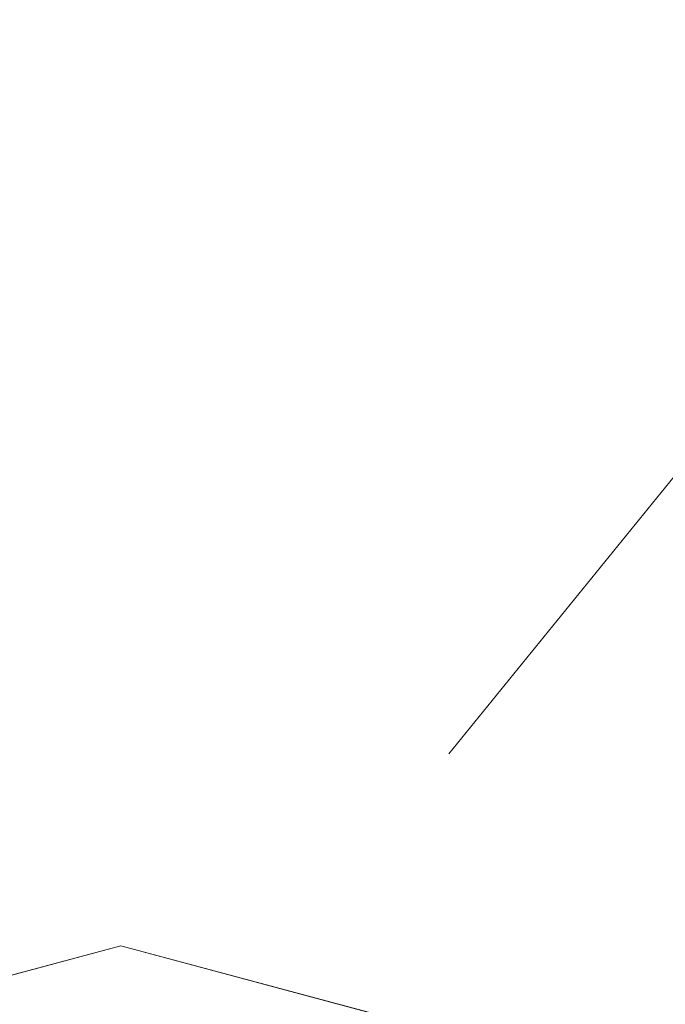
# Model space of a CAD drawing. Units: inches. Extents: x 375 to 1122, y 27 to 1069.
# Tile 89 of 155: x 725.203 to 728.243, y 859.033 to 863.668. Entities that reach past the tile are written whole.
import ezdxf

# ---------------------------------------------------------------- set-up
doc = ezdxf.new("R2010")
doc.units = ezdxf.units.IN
doc.layers.add('A-ANNO-DIMS', color=2, linetype='Continuous', lineweight=18)
doc.layers.add('Furniture', color=30, linetype='Continuous', lineweight=18)
doc.styles.get("Standard").update_dxf_attribs({"font": 'arial.ttf'})
doc.dimstyles.new('ISO-25', dxfattribs={"dimtxt": 12, "dimasz": 2.5, "dimexe": 1.5, "dimexo": 1.5, "dimtad": 1, "dimdec": 1, "dimlunit": 3, "dimtxsty": 'Standard', "dimblk": 'ARCHTICK', "dimcen": 2.5, "dimadec": 0, "dimazin": 0, "dimtfac": 1, "dimtdec": 1, "dimtmove": 0, "dimatfit": 3, "dimfxl": 1.5, "dimfxlon": 1, "dimarcsym": 0})

# ---------------------------------------------------------------- blocks, each defined once
blk = doc.blocks.new('A$C403C54AD')
blk.add_line((1.78922, 1.18993, 0.03663), (1.95298, 1.05694, 0.03663))
at = {"linetype": 'ByBlock', "invisible_edges": 5}
for points in [[(1.99415, 1.08761, -0.03783), (2.01014, 1.07837, -0.03783), (1.99406, 1.01834, -0.03783), (1.97559, 1.01834, -0.03783)], [(2.02347, 1.07068, -0.05168), (1.99415, 1.08761, -0.04244), (1.97559, 1.01834, -0.04244), (2.00945, 1.01834, -0.05168)], [(1.97559, 1.01834, -0.03783), (1.99406, 1.01834, -0.03783), (2.01014, 0.95832, -0.03783), (1.99415, 0.94908, -0.03783)], [(2.00945, 1.01834, -0.05168), (1.97559, 1.01834, -0.04244), (1.99415, 0.94908, -0.04244), (2.02347, 0.96601, -0.05168)]]:
    blk.add_3dface(points, dxfattribs=at)
at = {"linetype": 'ByBlock'}
for points in [[(1.99415, 1.08761, -0.04244), (1.99415, 1.08761, -0.03783), (1.97559, 1.01834, -0.03783), (1.97559, 1.01834, -0.04244)], [(1.97559, 1.01834, -0.04244), (1.97559, 1.01834, -0.03783), (1.99415, 0.94908, -0.03783), (1.99415, 0.94908, -0.04244)]]:
    blk.add_3dface(points, dxfattribs=at)
blk = doc.blocks.new('_ArchTick')
at = {"color": 0, "linetype": 'ByBlock', "const_width": 0.15}
blk.add_lwpolyline([(-0.5, -0.5), (0.5, 0.5)], dxfattribs=at)
blk = doc.blocks.new('*D85')
at = {"layer": 'A-ANNO-DIMS', "color": 0, "lineweight": -2, "transparency": 16777216}
for p, q in [((401.5073, 868.5277), (398.5073, 868.5277)), ((400.0073, 814.5277), (400.0073, 868.5277)), ((401.5073, 814.5277), (398.5073, 814.5277))]:
    blk.add_line(p, q, dxfattribs=at)
at = {"layer": 'Defpoints', "color": 0, "transparency": 16777216}
for p in [(400.0073, 868.5277), (845.0073, 868.5277), (845.0073, 814.5277)]:
    blk.add_point(p, dxfattribs=at)
at = {"layer": 'A-ANNO-DIMS', "color": 0, "lineweight": -2, "transparency": 16777216, "xscale": 2.5, "yscale": 2.5, "zscale": 2.5}
for p, rotation in [((400.0073, 868.5277), 90), ((400.0073, 814.5277), 270)]:
    blk.add_blockref('_ArchTick', p, dxfattribs=dict(at, rotation=rotation))
at = {"layer": 'A-ANNO-DIMS', "color": 0, "transparency": 16777216, "insert": (393.2555, 841.5277), "char_height": 12, "attachment_point": 5, "rotation": 90}
blk.add_mtext('4\'-6"', dxfattribs=at)
blk = doc.blocks.new('*D91')
at = {"layer": 'A-ANNO-DIMS', "color": 0, "lineweight": -2, "transparency": 16777216}
for p, q in [((728.0073, 1052.5277), (728.0073, 1055.5277)), ((788.0073, 1052.5277), (788.0073, 1055.5277)), ((728.0073, 1054.0277), (788.0073, 1054.0277))]:
    blk.add_line(p, q, dxfattribs=at)
at = {"layer": 'Defpoints', "color": 0, "transparency": 16777216}
for p in [(788.0073, 1054.0277), (728.0073, 774.0277), (788.0073, 774.0277)]:
    blk.add_point(p, dxfattribs=at)
at = {"layer": 'A-ANNO-DIMS', "color": 0, "lineweight": -2, "transparency": 16777216, "xscale": 2.5, "yscale": 2.5, "zscale": 2.5, "rotation": 180}
blk.add_blockref('_ArchTick', (728.0073, 1054.0277), dxfattribs=at)
at = {"layer": 'A-ANNO-DIMS', "color": 0, "lineweight": -2, "transparency": 16777216, "xscale": 2.5, "yscale": 2.5, "zscale": 2.5}
blk.add_blockref('_ArchTick', (788.0073, 1054.0277), dxfattribs=at)
at = {"layer": 'A-ANNO-DIMS', "color": 0, "transparency": 16777216, "insert": (758.0073, 1060.7796), "char_height": 12, "attachment_point": 5}
blk.add_mtext('5\'-0"', dxfattribs=at)

msp = doc.modelspace()

# ---------------------------------------------------------------- block references
at = {"layer": 'Furniture', "xscale": 39.9918517141215, "yscale": 39.9918517141215, "zscale": 39.9918517141215, "rotation": 270}
msp.add_blockref('A$C403C54AD', (684.9549, 938.3156, 0.024), dxfattribs=at)

# ---------------------------------------------------------------- dimensions: what is measured, and where the dimension line sits
at = {"layer": 'A-ANNO-DIMS'}
dim = msp.add_linear_dim(base=(788.0073, 1054.0277), p1=(728.0073, 774.0277), p2=(788.0073, 774.0277), dimstyle='ISO-25', override={"dimdec": 1, "dimlfac": 1, "dimrnd": 0, "dimzin": 1, "dimdsep": 46, "dimlunit": 4, "dimfrac": 2}, dxfattribs=at)
dim.commit()
dim.dimension.update_dxf_attribs({"geometry": '*D91', "text_midpoint": (758.0073, 1060.7796)})
dim = msp.add_linear_dim(base=(400.0073, 868.5277), p1=(845.0073, 814.5277), p2=(845.0073, 868.5277), angle=90, dimstyle='ISO-25', override={"dimdec": 1, "dimlfac": 1, "dimrnd": 0, "dimzin": 1, "dimdsep": 46, "dimlunit": 4, "dimfrac": 2}, dxfattribs=at)
dim.commit()
dim.dimension.update_dxf_attribs({"geometry": '*D85', "text_midpoint": (393.2555, 841.5277)})

doc.saveas('drawing.dxf')
